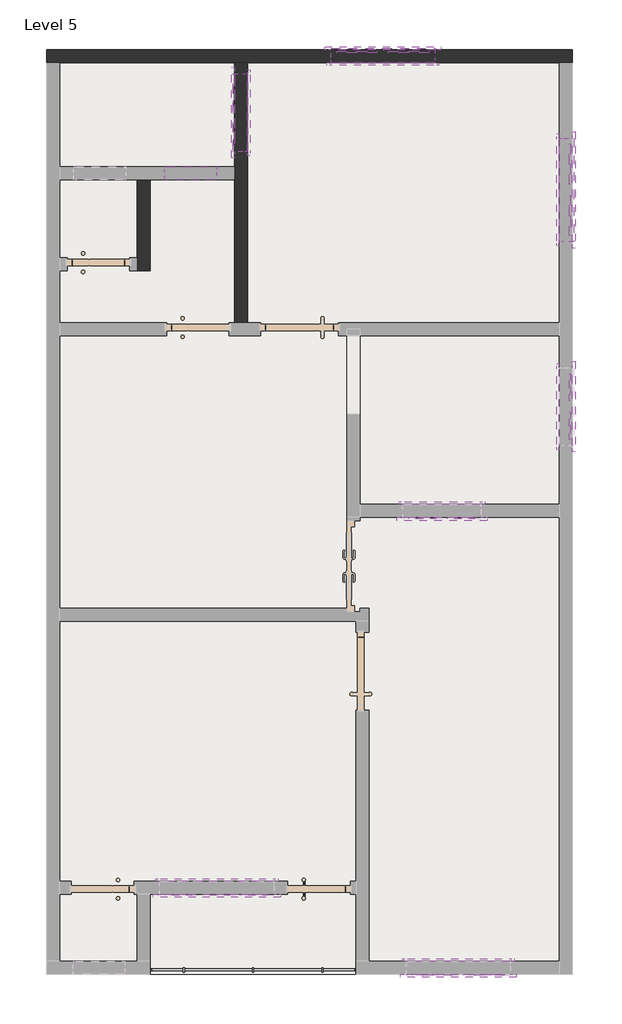
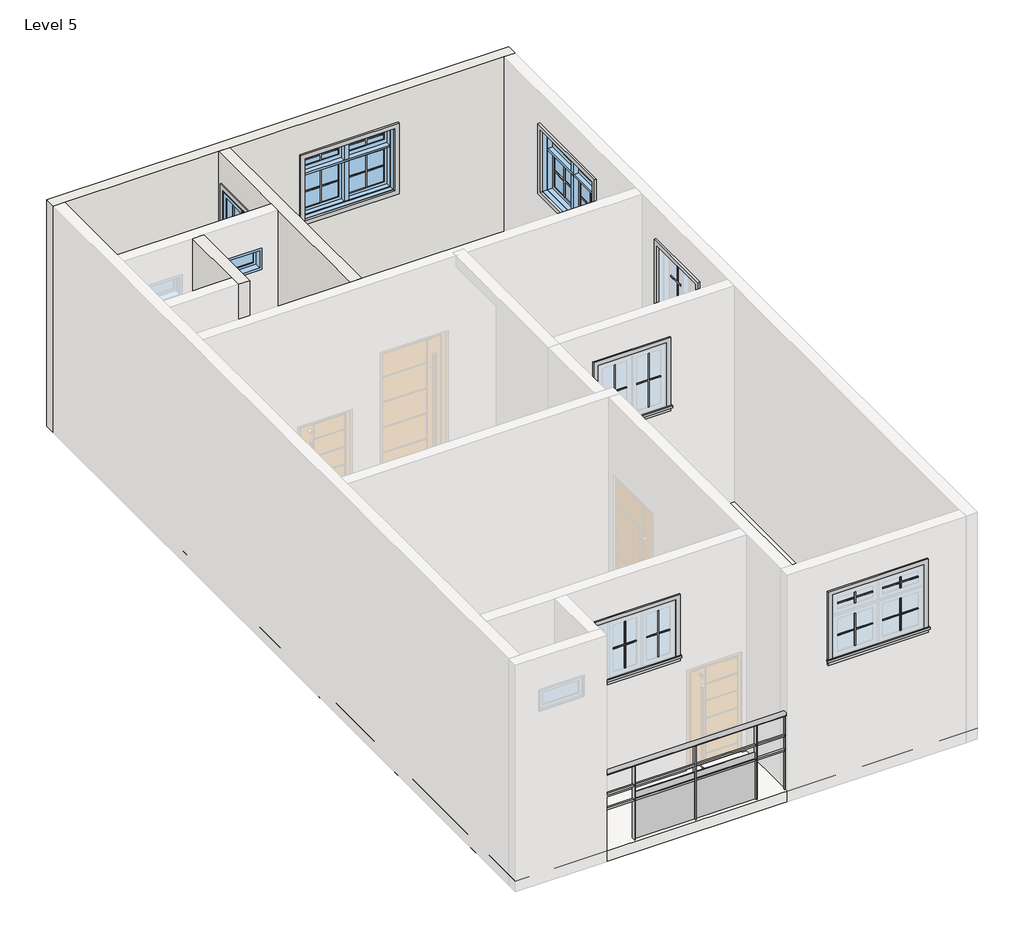
# One storey, part 2 of 2: 35 proxies, 4 windows, 3 walls, 1 railing, 1 slab.
"""IFC4 building model written with IfcOpenShell, lengths in millimetres."""

from ifc_helpers import new_model, si_unit, point, frame, origin, place, context, project, spatial, polyline, ellipse_curve, trimmed, outline, extrude, faceted_brep, transform, mapped, element, save
from ifc_brep_helpers import plane_surface, extruded_surface, advanced_brep
from components import m_muntin_pattern_2x2_m_muntin_pattern_2x2_ec2ff75e, m_muntin_pattern_2x2_m_muntin_pattern_2x2_6a19bea2, m_muntin_pattern_2x2_m_muntin_pattern_2x2_383df7b3, m_muntin_pattern_2x2_m_muntin_pattern_2x2_55460d9e, m_muntin_pattern_2x2_m_muntin_pattern_2x2_a9b7b7a9, m_muntin_pattern_2x2_m_muntin_pattern_2x2_c959817e, m_muntin_pattern_2x2_m_muntin_pattern_2x2_9259c5e2, m_trim_window_exterior_flat_with_sill_b1b88069, m_trim_window_exterior_flat_with_sill_8fa486dc, m_trim_window_exterior_flat_with_sill_2a9c44ae, m_trim_window_interior_flat_picture_frame_7d12f20c, m_trim_window_interior_flat_picture_frame_b6dd03a6, m_trim_window_interior_flat_picture_frame_c139440e, fixed_2_65c13adb, m_window_casement_double_3_e0bd8fa3, m_window_casement_double_awning_double_4_7efa9bbd

model = new_model("IFC4")

# Units and contexts
model_context = context("Model", 3, world=origin())
ifc_project = project(units=[si_unit("LENGTHUNIT", "METRE", prefix="MILLI")], contexts=[model_context])

# Site, building, storey
site = spatial("IfcSite", under=ifc_project)
building = spatial("IfcBuilding", under=site)
storey = spatial("IfcBuildingStorey", under=building, Name="Level 5", Elevation=3810.0)

# Proxies
placement = place(None, origin())
m_muntin_pattern_2x2_m_muntin_pattern_2x2_shape = m_muntin_pattern_2x2_m_muntin_pattern_2x2_ec2ff75e(model_context)
element("IfcBuildingElementProxy", 1, Name="M_Muntin Pattern_2x2 : M_Muntin Pattern_2x2", ObjectType="M_Muntin Pattern_2x2 : M_Muntin Pattern_2x2", at=placement, inside=storey, context=model_context, shape_type="MappedRepresentation", body=[
    mapped(m_muntin_pattern_2x2_m_muntin_pattern_2x2_shape, transform((-20164.8088079, 6316.5492053, 5708.65), x_axis=(1.0, 0.0, 0.0), y_axis=(0.0, 1.0, 0.0), z_axis=(0.0, 0.0, 1.0))),
])
element("IfcBuildingElementProxy", 2, Name="M_Muntin Pattern_2x2 : M_Muntin Pattern_2x2", ObjectType="M_Muntin Pattern_2x2 : M_Muntin Pattern_2x2", at=placement, inside=storey, context=model_context, shape_type="MappedRepresentation", body=[
    mapped(m_muntin_pattern_2x2_m_muntin_pattern_2x2_shape, transform((-17648.6213079, 4984.6367053, 5708.65), x_axis=(0.0, -1.0, 0.0), y_axis=(1.0, 0.0, 0.0), z_axis=(0.0, 0.0, 1.0))),
])
element("IfcBuildingElementProxy", 3, Name="M_Muntin Pattern_2x2 : M_Muntin Pattern_2x2", ObjectType="M_Muntin Pattern_2x2 : M_Muntin Pattern_2x2", at=placement, inside=storey, context=model_context, shape_type="MappedRepresentation", body=[
    mapped(m_muntin_pattern_2x2_m_muntin_pattern_2x2_shape, transform((-18672.7572454, -4510.2007947, 5708.65), x_axis=(-1.0, 0.0, 0.0), y_axis=(0.0, -1.0, 0.0), z_axis=(0.0, 0.0, 1.0))),
])
m_muntin_pattern_2x2_m_muntin_pattern_2x2_2_shape = m_muntin_pattern_2x2_m_muntin_pattern_2x2_6a19bea2(model_context)
element("IfcBuildingElementProxy", 4, Name="M_Muntin Pattern_2x2 : M_Muntin Pattern_2x2", ObjectType="M_Muntin Pattern_2x2 : M_Muntin Pattern_2x2", at=placement, inside=storey, context=model_context, shape_type="MappedRepresentation", body=[
    mapped(m_muntin_pattern_2x2_m_muntin_pattern_2x2_2_shape, transform((-19558.3838079, 6316.5492053, 5708.65), x_axis=(-1.0, 0.0, 0.0), y_axis=(0.0, -1.0, 0.0), z_axis=(0.0, 0.0, 1.0))),
])
element("IfcBuildingElementProxy", 5, Name="M_Muntin Pattern_2x2 : M_Muntin Pattern_2x2", ObjectType="M_Muntin Pattern_2x2 : M_Muntin Pattern_2x2", at=placement, inside=storey, context=model_context, shape_type="MappedRepresentation", body=[
    mapped(m_muntin_pattern_2x2_m_muntin_pattern_2x2_2_shape, transform((-17648.6213079, 4378.2117053, 5708.65), x_axis=(0.0, 1.0, 0.0), y_axis=(-1.0, 0.0, 0.0), z_axis=(0.0, 0.0, 1.0))),
])
element("IfcBuildingElementProxy", 6, Name="M_Muntin Pattern_2x2 : M_Muntin Pattern_2x2", ObjectType="M_Muntin Pattern_2x2 : M_Muntin Pattern_2x2", at=placement, inside=storey, context=model_context, shape_type="MappedRepresentation", body=[
    mapped(m_muntin_pattern_2x2_m_muntin_pattern_2x2_2_shape, transform((-19279.1822454, -4510.2007947, 5708.65), x_axis=(1.0, 0.0, 0.0), y_axis=(0.0, 1.0, 0.0), z_axis=(0.0, 0.0, 1.0))),
])
m_muntin_pattern_2x2_m_muntin_pattern_2x2_3_shape = m_muntin_pattern_2x2_m_muntin_pattern_2x2_383df7b3(model_context)
element("IfcBuildingElementProxy", 7, Name="M_Muntin Pattern_2x2 : M_Muntin Pattern_2x2", ObjectType="M_Muntin Pattern_2x2 : M_Muntin Pattern_2x2", at=placement, inside=storey, context=model_context, shape_type="MappedRepresentation", body=[
    mapped(m_muntin_pattern_2x2_m_muntin_pattern_2x2_3_shape, transform((-19558.3838079, 6316.5492053, 6308.65), x_axis=(-1.0, 0.0, 0.0), y_axis=(0.0, -1.0, 0.0), z_axis=(0.0, 0.0, 1.0))),
])
element("IfcBuildingElementProxy", 8, Name="M_Muntin Pattern_2x2 : M_Muntin Pattern_2x2", ObjectType="M_Muntin Pattern_2x2 : M_Muntin Pattern_2x2", at=placement, inside=storey, context=model_context, shape_type="MappedRepresentation", body=[
    mapped(m_muntin_pattern_2x2_m_muntin_pattern_2x2_3_shape, transform((-20164.8088079, 6316.5492053, 6308.65), x_axis=(-1.0, 0.0, 0.0), y_axis=(0.0, -1.0, 0.0), z_axis=(0.0, 0.0, 1.0))),
])
element("IfcBuildingElementProxy", 9, Name="M_Muntin Pattern_2x2 : M_Muntin Pattern_2x2", ObjectType="M_Muntin Pattern_2x2 : M_Muntin Pattern_2x2", at=placement, inside=storey, context=model_context, shape_type="MappedRepresentation", body=[
    mapped(m_muntin_pattern_2x2_m_muntin_pattern_2x2_3_shape, transform((-17648.6213079, 4378.2117053, 6308.65), x_axis=(0.0, 1.0, 0.0), y_axis=(-1.0, 0.0, 0.0), z_axis=(0.0, 0.0, 1.0))),
])
element("IfcBuildingElementProxy", 10, Name="M_Muntin Pattern_2x2 : M_Muntin Pattern_2x2", ObjectType="M_Muntin Pattern_2x2 : M_Muntin Pattern_2x2", at=placement, inside=storey, context=model_context, shape_type="MappedRepresentation", body=[
    mapped(m_muntin_pattern_2x2_m_muntin_pattern_2x2_3_shape, transform((-17648.6213079, 4984.6367053, 6308.65), x_axis=(0.0, 1.0, 0.0), y_axis=(-1.0, 0.0, 0.0), z_axis=(0.0, 0.0, 1.0))),
])
element("IfcBuildingElementProxy", 11, Name="M_Muntin Pattern_2x2 : M_Muntin Pattern_2x2", ObjectType="M_Muntin Pattern_2x2 : M_Muntin Pattern_2x2", at=placement, inside=storey, context=model_context, shape_type="MappedRepresentation", body=[
    mapped(m_muntin_pattern_2x2_m_muntin_pattern_2x2_3_shape, transform((-19279.1822454, -4510.2007947, 6308.65), x_axis=(1.0, 0.0, 0.0), y_axis=(0.0, 1.0, 0.0), z_axis=(0.0, 0.0, 1.0))),
])
element("IfcBuildingElementProxy", 12, Name="M_Muntin Pattern_2x2 : M_Muntin Pattern_2x2", ObjectType="M_Muntin Pattern_2x2 : M_Muntin Pattern_2x2", at=placement, inside=storey, context=model_context, shape_type="MappedRepresentation", body=[
    mapped(m_muntin_pattern_2x2_m_muntin_pattern_2x2_3_shape, transform((-18672.7572454, -4510.2007947, 6308.65), x_axis=(1.0, 0.0, 0.0), y_axis=(0.0, 1.0, 0.0), z_axis=(0.0, 0.0, 1.0))),
])
m_muntin_pattern_2x2_m_muntin_pattern_2x2_4_shape = m_muntin_pattern_2x2_m_muntin_pattern_2x2_55460d9e(model_context)
element("IfcBuildingElementProxy", 13, Name="M_Muntin Pattern_2x2 : M_Muntin Pattern_2x2", ObjectType="M_Muntin Pattern_2x2 : M_Muntin Pattern_2x2", at=placement, inside=storey, context=model_context, shape_type="MappedRepresentation", body=[
    mapped(m_muntin_pattern_2x2_m_muntin_pattern_2x2_4_shape, transform((-18939.9533391, 849.1992053, 5708.65), x_axis=(-1.0, 0.0, 0.0), y_axis=(0.0, -1.0, 0.0), z_axis=(0.0, 0.0, 1.0))),
])
element("IfcBuildingElementProxy", 14, Name="M_Muntin Pattern_2x2 : M_Muntin Pattern_2x2", ObjectType="M_Muntin Pattern_2x2 : M_Muntin Pattern_2x2", at=placement, inside=storey, context=model_context, shape_type="MappedRepresentation", body=[
    mapped(m_muntin_pattern_2x2_m_muntin_pattern_2x2_4_shape, transform((-17648.6213079, 2366.8492053, 5708.65), x_axis=(0.0, -1.0, 0.0), y_axis=(1.0, 0.0, 0.0), z_axis=(0.0, 0.0, 1.0))),
])
element("IfcBuildingElementProxy", 15, Name="M_Muntin Pattern_2x2 : M_Muntin Pattern_2x2", ObjectType="M_Muntin Pattern_2x2 : M_Muntin Pattern_2x2", at=placement, inside=storey, context=model_context, shape_type="MappedRepresentation", body=[
    mapped(m_muntin_pattern_2x2_m_muntin_pattern_2x2_4_shape, transform((-21591.9713079, 5362.4617053, 5708.65), x_axis=(0.0, 1.0, 0.0), y_axis=(-1.0, 0.0, 0.0), z_axis=(0.0, 0.0, 1.0))),
])
m_muntin_pattern_2x2_m_muntin_pattern_2x2_5_shape = m_muntin_pattern_2x2_m_muntin_pattern_2x2_a9b7b7a9(model_context)
element("IfcBuildingElementProxy", 16, Name="M_Muntin Pattern_2x2 : M_Muntin Pattern_2x2", ObjectType="M_Muntin Pattern_2x2 : M_Muntin Pattern_2x2", at=placement, inside=storey, context=model_context, shape_type="MappedRepresentation", body=[
    mapped(m_muntin_pattern_2x2_m_muntin_pattern_2x2_5_shape, transform((-19393.9783391, 849.1992053, 5708.65), x_axis=(1.0, 0.0, 0.0), y_axis=(0.0, 1.0, 0.0), z_axis=(0.0, 0.0, 1.0))),
])
element("IfcBuildingElementProxy", 17, Name="M_Muntin Pattern_2x2 : M_Muntin Pattern_2x2", ObjectType="M_Muntin Pattern_2x2 : M_Muntin Pattern_2x2", at=placement, inside=storey, context=model_context, shape_type="MappedRepresentation", body=[
    mapped(m_muntin_pattern_2x2_m_muntin_pattern_2x2_5_shape, transform((-17648.6213079, 1912.8242053, 5708.65), x_axis=(0.0, 1.0, 0.0), y_axis=(-1.0, 0.0, 0.0), z_axis=(0.0, 0.0, 1.0))),
])
element("IfcBuildingElementProxy", 18, Name="M_Muntin Pattern_2x2 : M_Muntin Pattern_2x2", ObjectType="M_Muntin Pattern_2x2 : M_Muntin Pattern_2x2", at=placement, inside=storey, context=model_context, shape_type="MappedRepresentation", body=[
    mapped(m_muntin_pattern_2x2_m_muntin_pattern_2x2_5_shape, transform((-21591.9713079, 5816.4867053, 5708.65), x_axis=(0.0, -1.0, 0.0), y_axis=(1.0, 0.0, 0.0), z_axis=(0.0, 0.0, 1.0))),
])
m_muntin_pattern_2x2_m_muntin_pattern_2x2_6_shape = m_muntin_pattern_2x2_m_muntin_pattern_2x2_c959817e(model_context)
element("IfcBuildingElementProxy", 19, Name="M_Muntin Pattern_2x2 : M_Muntin Pattern_2x2", ObjectType="M_Muntin Pattern_2x2 : M_Muntin Pattern_2x2", at=placement, inside=storey, context=model_context, shape_type="MappedRepresentation", body=[
    mapped(m_muntin_pattern_2x2_m_muntin_pattern_2x2_6_shape, transform((-21364.4296412, -3570.4007947, 5708.65), x_axis=(-1.0, 0.0, 0.0), y_axis=(0.0, -1.0, 0.0), z_axis=(0.0, 0.0, 1.0))),
])
m_muntin_pattern_2x2_m_muntin_pattern_2x2_7_shape = m_muntin_pattern_2x2_m_muntin_pattern_2x2_9259c5e2(model_context)
element("IfcBuildingElementProxy", 20, Name="M_Muntin Pattern_2x2 : M_Muntin Pattern_2x2", ObjectType="M_Muntin Pattern_2x2 : M_Muntin Pattern_2x2", at=placement, inside=storey, context=model_context, shape_type="MappedRepresentation", body=[
    mapped(m_muntin_pattern_2x2_m_muntin_pattern_2x2_7_shape, transform((-22257.6629746, -3570.4007947, 5708.65), x_axis=(1.0, 0.0, 0.0), y_axis=(0.0, 1.0, 0.0), z_axis=(0.0, 0.0, 1.0))),
])
element("IfcBuildingElementProxy", 21, Name="M_Muntin Pattern_2x2 : M_Muntin Pattern_2x2", ObjectType="M_Muntin Pattern_2x2 : M_Muntin Pattern_2x2", at=placement, inside=storey, context=model_context, shape_type="MappedRepresentation", body=[
    mapped(m_muntin_pattern_2x2_m_muntin_pattern_2x2_7_shape, transform((-21811.0463079, -3570.4007947, 5708.65), x_axis=(1.0, 0.0, 0.0), y_axis=(0.0, 1.0, 0.0), z_axis=(0.0, 0.0, 1.0))),
])
m_trim_window_exterior_flat_with_sill_shape = m_trim_window_exterior_flat_with_sill_b1b88069(model_context)
element("IfcBuildingElementProxy", 22, Name="M_Trim-Window-Exterior-Flat : with Sill", ObjectType="M_Trim-Window-Exterior-Flat : with Sill", at=placement, inside=storey, context=model_context, shape_type="MappedRepresentation", body=[
    mapped(m_trim_window_exterior_flat_with_sill_shape, transform((-19861.5963079, 6326.0742053, 6538.8), x_axis=(-1.0, 0.0, 0.0), y_axis=(0.0, 0.0, 1.0), z_axis=(0.0, 1.0, 0.0))),
])
element("IfcBuildingElementProxy", 23, Name="M_Trim-Window-Exterior-Flat : with Sill", ObjectType="M_Trim-Window-Exterior-Flat : with Sill", at=placement, inside=storey, context=model_context, shape_type="MappedRepresentation", body=[
    mapped(m_trim_window_exterior_flat_with_sill_shape, transform((-17639.0963079, 4681.4242053, 6538.8), x_axis=(0.0, 1.0, 0.0), y_axis=(0.0, 0.0, 1.0), z_axis=(1.0, 0.0, 0.0))),
])
element("IfcBuildingElementProxy", 24, Name="M_Trim-Window-Exterior-Flat : with Sill", ObjectType="M_Trim-Window-Exterior-Flat : with Sill", at=placement, inside=storey, context=model_context, shape_type="MappedRepresentation", body=[
    mapped(m_trim_window_exterior_flat_with_sill_shape, transform((-18975.9697454, -4519.7257947, 6538.8), x_axis=(1.0, 0.0, 0.0), y_axis=(0.0, 0.0, 1.0), z_axis=(0.0, -1.0, 0.0))),
])
m_trim_window_exterior_flat_with_sill_2_shape = m_trim_window_exterior_flat_with_sill_8fa486dc(model_context)
element("IfcBuildingElementProxy", 25, Name="M_Trim-Window-Exterior-Flat : with Sill", ObjectType="M_Trim-Window-Exterior-Flat : with Sill", at=placement, inside=storey, context=model_context, shape_type="MappedRepresentation", body=[
    mapped(m_trim_window_exterior_flat_with_sill_2_shape, transform((-19166.9658391, 839.6742053, 6538.8), x_axis=(1.0, 0.0, 0.0), y_axis=(0.0, 0.0, 1.0), z_axis=(0.0, -1.0, 0.0))),
])
element("IfcBuildingElementProxy", 26, Name="M_Trim-Window-Exterior-Flat : with Sill", ObjectType="M_Trim-Window-Exterior-Flat : with Sill", at=placement, inside=storey, context=model_context, shape_type="MappedRepresentation", body=[
    mapped(m_trim_window_exterior_flat_with_sill_2_shape, transform((-17639.0963079, 2139.8367053, 6538.8), x_axis=(0.0, 1.0, 0.0), y_axis=(0.0, 0.0, 1.0), z_axis=(1.0, 0.0, 0.0))),
])
element("IfcBuildingElementProxy", 27, Name="M_Trim-Window-Exterior-Flat : with Sill", ObjectType="M_Trim-Window-Exterior-Flat : with Sill", at=placement, inside=storey, context=model_context, shape_type="MappedRepresentation", body=[
    mapped(m_trim_window_exterior_flat_with_sill_2_shape, transform((-21601.4963079, 5589.4742053, 6538.8), x_axis=(0.0, -1.0, 0.0), y_axis=(0.0, 0.0, 1.0), z_axis=(-1.0, 0.0, 0.0))),
])
m_trim_window_exterior_flat_with_sill_3_shape = m_trim_window_exterior_flat_with_sill_2a9c44ae(model_context)
element("IfcBuildingElementProxy", 28, Name="M_Trim-Window-Exterior-Flat : with Sill", ObjectType="M_Trim-Window-Exterior-Flat : with Sill", at=placement, inside=storey, context=model_context, shape_type="MappedRepresentation", body=[
    mapped(m_trim_window_exterior_flat_with_sill_3_shape, transform((-21811.0463079, -3579.9257947, 6438.8), x_axis=(1.0, 0.0, 0.0), y_axis=(0.0, 0.0, 1.0), z_axis=(0.0, -1.0, 0.0))),
])
m_trim_window_interior_flat_picture_frame_shape = m_trim_window_interior_flat_picture_frame_7d12f20c(model_context)
element("IfcBuildingElementProxy", 29, Name="M_Trim-Window-Interior-Flat : Picture Frame", ObjectType="M_Trim-Window-Interior-Flat : Picture Frame", at=placement, inside=storey, context=model_context, shape_type="MappedRepresentation", body=[
    mapped(m_trim_window_interior_flat_picture_frame_shape, transform((-19861.5963079, 6173.6742053, 6538.8), x_axis=(1.0, 0.0, 0.0), y_axis=(0.0, 0.0, 1.0), z_axis=(0.0, -1.0, 0.0))),
])
element("IfcBuildingElementProxy", 30, Name="M_Trim-Window-Interior-Flat : Picture Frame", ObjectType="M_Trim-Window-Interior-Flat : Picture Frame", at=placement, inside=storey, context=model_context, shape_type="MappedRepresentation", body=[
    mapped(m_trim_window_interior_flat_picture_frame_shape, transform((-17791.4963079, 4681.4242053, 6538.8), x_axis=(0.0, -1.0, 0.0), y_axis=(0.0, 0.0, 1.0), z_axis=(-1.0, 0.0, 0.0))),
])
element("IfcBuildingElementProxy", 31, Name="M_Trim-Window-Interior-Flat : Picture Frame", ObjectType="M_Trim-Window-Interior-Flat : Picture Frame", at=placement, inside=storey, context=model_context, shape_type="MappedRepresentation", body=[
    mapped(m_trim_window_interior_flat_picture_frame_shape, transform((-18975.9697454, -4367.3257947, 6538.8), x_axis=(-1.0, 0.0, 0.0), y_axis=(0.0, 0.0, 1.0), z_axis=(0.0, 1.0, 0.0))),
])
m_trim_window_interior_flat_picture_frame_2_shape = m_trim_window_interior_flat_picture_frame_b6dd03a6(model_context)
element("IfcBuildingElementProxy", 32, Name="M_Trim-Window-Interior-Flat : Picture Frame", ObjectType="M_Trim-Window-Interior-Flat : Picture Frame", at=placement, inside=storey, context=model_context, shape_type="MappedRepresentation", body=[
    mapped(m_trim_window_interior_flat_picture_frame_2_shape, transform((-19166.9658391, 992.0742053, 6538.8), x_axis=(-1.0, 0.0, 0.0), y_axis=(0.0, 0.0, 1.0), z_axis=(0.0, 1.0, 0.0))),
])
element("IfcBuildingElementProxy", 33, Name="M_Trim-Window-Interior-Flat : Picture Frame", ObjectType="M_Trim-Window-Interior-Flat : Picture Frame", at=placement, inside=storey, context=model_context, shape_type="MappedRepresentation", body=[
    mapped(m_trim_window_interior_flat_picture_frame_2_shape, transform((-17791.4963079, 2139.8367053, 6538.8), x_axis=(0.0, -1.0, 0.0), y_axis=(0.0, 0.0, 1.0), z_axis=(-1.0, 0.0, 0.0))),
])
element("IfcBuildingElementProxy", 34, Name="M_Trim-Window-Interior-Flat : Picture Frame", ObjectType="M_Trim-Window-Interior-Flat : Picture Frame", at=placement, inside=storey, context=model_context, shape_type="MappedRepresentation", body=[
    mapped(m_trim_window_interior_flat_picture_frame_2_shape, transform((-21449.0963079, 5589.4742053, 6538.8), x_axis=(0.0, 1.0, 0.0), y_axis=(0.0, 0.0, 1.0), z_axis=(1.0, 0.0, 0.0))),
])
m_trim_window_interior_flat_picture_frame_3_shape = m_trim_window_interior_flat_picture_frame_c139440e(model_context)
element("IfcBuildingElementProxy", 35, Name="M_Trim-Window-Interior-Flat : Picture Frame", ObjectType="M_Trim-Window-Interior-Flat : Picture Frame", at=placement, inside=storey, context=model_context, shape_type="MappedRepresentation", body=[
    mapped(m_trim_window_interior_flat_picture_frame_3_shape, transform((-21811.0463079, -3427.5257947, 6438.8), x_axis=(-1.0, 0.0, 0.0), y_axis=(0.0, 0.0, 1.0), z_axis=(0.0, 1.0, 0.0))),
])

# Railing
element("IfcRailing", 36, ObjectType="Glass Panel - Bottom Fill", at=placement, inside=storey, context=model_context, shape_type="SolidModel", body=[
    advanced_brep(
    [(-22592.0963079, -4430.8257947, 5029.2), (-22592.0963079, -4507.0257947, 5029.2), (-20179.0963079, -4430.8257947, 5029.2), (-20179.0963079, -4507.0257947, 5029.2)],
    [
        (0, 1, ellipse_curve(frame((-22592.0963079, -4468.9257947, 5029.2), z_axis=(-1.0, 0.0, 0.0), x_axis=(0.0, -1.0, 0.0)), 38.1, 28.575)),
        (1, 0, ellipse_curve(frame((-22592.0963079, -4468.9257947, 5029.2), z_axis=(-1.0, 0.0, 0.0), x_axis=(0.0, -1.0, 0.0)), 38.1, 28.575)),
        (2, 3, ellipse_curve(frame((-20179.0963079, -4468.9257947, 5029.2), z_axis=(1.0, 0.0, 0.0), x_axis=(0.0, -1.0, 0.0)), 38.1, 28.575)),
        (3, 2, ellipse_curve(frame((-20179.0963079, -4468.9257947, 5029.2), z_axis=(1.0, 0.0, 0.0), x_axis=(0.0, -1.0, 0.0)), 38.1, 28.575)),
        (0, 2),
        (3, 1),
    ],
    [
        plane_surface(frame((-22592.0963079, -4468.9257947, 5029.2), z_axis=(-1.0, 0.0, 0.0), x_axis=(0.0, 1.0, 0.0))),
        plane_surface(frame((-20179.0963079, -4468.9257947, 5029.2), z_axis=(1.0, 0.0, 0.0), x_axis=(0.0, 1.0, 0.0))),
        extruded_surface(trimmed(ellipse_curve(frame((-20179.0963079, -4468.9257947, 5029.2), z_axis=(-1.0, 0.0, 0.0), x_axis=(0.0, -1.0, 0.0)), 38.1, 28.575), [point((-20179.0963079, -4430.8257947, 5029.2))], [point((-20179.0963079, -4507.0257947, 5029.2))], True, "CARTESIAN"), (-2413.0, 0.0, 0.0), 2413.0),
        extruded_surface(trimmed(ellipse_curve(frame((-20179.0963079, -4468.9257947, 5029.2), z_axis=(-1.0, 0.0, 0.0), x_axis=(0.0, -1.0, 0.0)), 38.1, 28.575), [point((-20179.0963079, -4507.0257947, 5029.2))], [point((-20179.0963079, -4430.8257947, 5029.2))], True, "CARTESIAN"), (-2413.0, 0.0, 0.0), 2413.0),
    ],
    [
        (0, [[1, 2]]),
        (1, [[3, 4]]),
        (2, [[-1, 5, -4, 6]]),
        (3, [[-2, -6, -3, -5]]),
    ],
),
    extrude(outline(polyline([(-22592.0963079, -4481.6257947), (-22592.0963079, -4456.2257947), (-20179.0963079, -4456.2257947), (-20179.0963079, -4481.6257947), (-22592.0963079, -4481.6257947)])), frame((0.0, 0.0, 4711.7), z_axis=(0.0, 0.0, 1.0), x_axis=(1.0, 0.0, 0.0)), (0.0, 0.0, 1.0), 25.4),
    extrude(outline(polyline([(-22592.0963079, -4481.6257947), (-22592.0963079, -4456.2257947), (-20179.0963079, -4456.2257947), (-20179.0963079, -4481.6257947), (-22592.0963079, -4481.6257947)])), frame((0.0, 0.0, 4508.5), z_axis=(0.0, 0.0, 1.0), x_axis=(1.0, 0.0, 0.0)), (0.0, 0.0, 1.0), 25.4),
    extrude(outline(polyline([(-20579.1463079, -4494.3257947), (-20579.1463079, -4443.5257947), (-20566.4463079, -4443.5257947), (-20566.4463079, -4494.3257947), (-20579.1463079, -4494.3257947)])), frame((0.0, 0.0, 3810.0), z_axis=(0.0, 0.0, 1.0), x_axis=(1.0, 0.0, 0.0)), (0.0, 0.0, 1.0), 1190.625),
    extrude(outline(polyline([(-21385.5963079, -4462.3906377), (-20572.7963079, -4462.3906377), (-20572.7963079, -4468.7406377), (-21385.5963079, -4468.7406377), (-21385.5963079, -4462.3906377)])), frame((0.0, 0.0, 3911.6), z_axis=(0.0, 0.0, 1.0), x_axis=(1.0, 0.0, 0.0)), (0.0, 0.0, 1.0), 711.2),
    extrude(outline(polyline([(-21391.9463079, -4494.3257947), (-21391.9463079, -4443.5257947), (-21379.2463079, -4443.5257947), (-21379.2463079, -4494.3257947), (-21391.9463079, -4494.3257947)])), frame((0.0, 0.0, 3810.0), z_axis=(0.0, 0.0, 1.0), x_axis=(1.0, 0.0, 0.0)), (0.0, 0.0, 1.0), 1190.625),
    extrude(outline(polyline([(-22198.3963079, -4462.3906377), (-21385.5963079, -4462.3906377), (-21385.5963079, -4468.7406377), (-22198.3963079, -4468.7406377), (-22198.3963079, -4462.3906377)])), frame((0.0, 0.0, 3911.6), z_axis=(0.0, 0.0, 1.0), x_axis=(1.0, 0.0, 0.0)), (0.0, 0.0, 1.0), 711.2),
    extrude(outline(polyline([(-22204.7463079, -4494.3257947), (-22204.7463079, -4443.5257947), (-22192.0463079, -4443.5257947), (-22192.0463079, -4494.3257947), (-22204.7463079, -4494.3257947)])), frame((0.0, 0.0, 3810.0), z_axis=(0.0, 0.0, 1.0), x_axis=(1.0, 0.0, 0.0)), (0.0, 0.0, 1.0), 1190.625),
    extrude(outline(polyline([(-20191.7963079, -4478.4507947), (-20191.7963079, -4459.4007947), (-20172.7463079, -4459.4007947), (-20172.7463079, -4478.4507947), (-20191.7963079, -4478.4507947)])), frame((0.0, 0.0, 3810.0), z_axis=(0.0, 0.0, 1.0), x_axis=(1.0, 0.0, 0.0)), (0.0, 0.0, 1.0), 1190.625),
    extrude(outline(polyline([(-22598.4463079, -4478.4507947), (-22598.4463079, -4459.4007947), (-22579.3963079, -4459.4007947), (-22579.3963079, -4478.4507947), (-22598.4463079, -4478.4507947)])), frame((0.0, 0.0, 3810.0), z_axis=(0.0, 0.0, 1.0), x_axis=(1.0, 0.0, 0.0)), (0.0, 0.0, 1.0), 1190.625),
])

# Slab
element("IfcSlab", 37, ObjectType="Generic - 6\"", at=placement, inside=storey, context=model_context, shape_type="SweptSolid", body=[
    extrude(outline(polyline([(-23811.2963079, -4519.7257947), (-23811.2963079, 6326.0742053), (-17639.0963079, 6326.0742053), (-17639.0963079, -4519.7257947), (-23811.2963079, -4519.7257947)])), frame((0.0, 0.0, 3810.0), z_axis=(0.0, 0.0, 1.0), x_axis=(1.0, 0.0, 0.0)), (0.0, 0.0, 1.0), 152.4),
])

# Walls
element("IfcWall", 38, ObjectType="Generic - 6\"", at=placement, inside=storey, context=model_context, shape_type="Brep", body=[
    faceted_brep([(-23811.2963079, 6173.6742053, 3810.0), (-23658.8963079, 6173.6742053, 3810.0), (-21601.4963079, 6173.6742053, 3810.0), (-21449.0963079, 6173.6742053, 3810.0), (-17791.4963079, 6173.6742053, 3810.0), (-17639.0963079, 6173.6742053, 3810.0), (-17639.0963079, 6173.6742053, 7010.4), (-17791.4963079, 6173.6742053, 7010.4), (-21449.0963079, 6173.6742053, 7010.4), (-21601.4963079, 6173.6742053, 7010.4), (-23658.8963079, 6173.6742053, 7010.4), (-23811.2963079, 6173.6742053, 7010.4), (-19251.9963079, 6173.6742053, 6538.8), (-19251.9963079, 6173.6742053, 5638.8), (-20471.1963079, 6173.6742053, 5638.8), (-20471.1963079, 6173.6742053, 6538.8), (-23811.2963079, 6326.0742053, 3810.0), (-23811.2963079, 6326.0742053, 7010.4), (-17639.0963079, 6326.0742053, 7010.4), (-17639.0963079, 6326.0742053, 3810.0), (-19251.9963079, 6326.0742053, 6538.8), (-20471.1963079, 6326.0742053, 6538.8), (-20471.1963079, 6326.0742053, 5638.8), (-19251.9963079, 6326.0742053, 5638.8)], [[[0, 1, 2, 3, 4, 5, 6, 7, 8, 9, 10, 11], [12, 13, 14, 15]], [[16, 17, 18, 19], [20, 21, 22, 23]], [[5, 4, 3, 2, 1, 0, 16, 19]], [[11, 10, 9, 8, 7, 6, 18, 17]], [[6, 5, 19, 18]], [[0, 11, 17, 16]], [[13, 12, 20, 23]], [[14, 13, 23, 22]], [[15, 14, 22, 21]], [[12, 15, 21, 20]]]),
])
element("IfcWall", 39, ObjectType="Generic - 6\"", at=placement, inside=storey, context=model_context, shape_type="Brep", body=[
    faceted_brep([(-21601.4963079, 6173.6742053, 3810.0), (-21601.4963079, 4954.4742053, 3810.0), (-21601.4963079, 4802.0742053, 3810.0), (-21601.4963079, 3125.6742053, 3810.0), (-21601.4963079, 3125.6742053, 7010.4), (-21601.4963079, 4802.0742053, 7010.4), (-21601.4963079, 4954.4742053, 7010.4), (-21601.4963079, 6173.6742053, 7010.4), (-21601.4963079, 6046.6742053, 6538.8), (-21601.4963079, 5132.2742053, 6538.8), (-21601.4963079, 5132.2742053, 5638.8), (-21601.4963079, 6046.6742053, 5638.8), (-21449.0963079, 6173.6742053, 3810.0), (-21449.0963079, 6173.6742053, 7010.4), (-21449.0963079, 3125.6742053, 7010.4), (-21449.0963079, 3125.6742053, 3810.0), (-21449.0963079, 6046.6742053, 6538.8), (-21449.0963079, 6046.6742053, 5638.8), (-21449.0963079, 5132.2742053, 5638.8), (-21449.0963079, 5132.2742053, 6538.8)], [[[0, 1, 2, 3, 4, 5, 6, 7], [8, 9, 10, 11]], [[12, 13, 14, 15], [16, 17, 18, 19]], [[3, 2, 1, 0, 12, 15]], [[7, 6, 5, 4, 14, 13]], [[0, 7, 13, 12]], [[4, 3, 15, 14]], [[17, 16, 8, 11]], [[18, 17, 11, 10]], [[19, 18, 10, 9]], [[16, 19, 9, 8]]]),
])
element("IfcWall", 40, ObjectType="Generic - 6\"", at=placement, inside=storey, context=model_context, shape_type="Brep", body=[
    faceted_brep([(-22744.4963079, 4802.0742053, 3810.0), (-22744.4963079, 3887.6742053, 3810.0), (-22744.4963079, 3735.2742053, 3810.0), (-22744.4963079, 3735.2742053, 7010.4), (-22744.4963079, 3887.6742053, 7010.4), (-22744.4963079, 4802.0742053, 7010.4), (-22592.0963079, 4802.0742053, 3810.0), (-22592.0963079, 4802.0742053, 7010.4), (-22592.0963079, 3735.2742053, 7010.4), (-22592.0963079, 3735.2742053, 3810.0)], [[[0, 1, 2, 3, 4, 5]], [[6, 7, 8, 9]], [[2, 1, 0, 6, 9]], [[5, 4, 3, 8, 7]], [[0, 5, 7, 6]], [[3, 2, 9, 8]]]),
])

# Windows
fixed_2_shape = fixed_2_65c13adb(model_context)
element("IfcWindow", 41, ObjectType="Fixed : 2'", at=placement, inside=storey, context=model_context, shape_type="MappedRepresentation", body=[
    mapped(fixed_2_shape, transform((-22079.3338079, 4878.2742053, 5334.0), x_axis=(1.0, 0.0, 0.0), y_axis=(0.0, 1.0, 0.0), z_axis=(0.0, 0.0, 1.0))),
])
m_window_casement_double_3_shape = m_window_casement_double_3_e0bd8fa3(model_context)
element("IfcWindow", 42, ObjectType="M_Window-Casement-Double : 3'", at=placement, inside=storey, context=model_context, shape_type="MappedRepresentation", body=[
    mapped(m_window_casement_double_3_shape, transform((-21525.2963079, 5589.4742053, 4738.8), x_axis=(0.0, 1.0, 0.0), y_axis=(-1.0, 0.0, 0.0), z_axis=(0.0, 0.0, 1.0))),
])
m_window_casement_double_awning_double_4_shape = m_window_casement_double_awning_double_4_7efa9bbd(model_context)
element("IfcWindow", 43, ObjectType="M_Window-Casement-Double-Awning-Double : 4'", at=placement, inside=storey, context=model_context, shape_type="MappedRepresentation", body=[
    mapped(m_window_casement_double_awning_double_4_shape, transform((-19861.5963079, 6249.8742053, 4738.8), x_axis=(1.0, 0.0, 0.0), y_axis=(0.0, 1.0, 0.0), z_axis=(0.0, 0.0, 1.0))),
])
element("IfcWindow", 44, ObjectType="M_Window-Casement-Double-Awning-Double : 4'", at=placement, inside=storey, context=model_context, shape_type="MappedRepresentation", body=[
    mapped(m_window_casement_double_awning_double_4_shape, transform((-17715.2963079, 4681.4242053, 4738.8), x_axis=(0.0, -1.0, 0.0), y_axis=(1.0, 0.0, 0.0), z_axis=(0.0, 0.0, 1.0))),
])

save(model, "model.ifc")

# Revit data of these elements
# Type "M_Muntin Pattern_2x2 : M_Muntin Pattern_2x2"
#   Width [instance default] = 3' - 11.24409"
#   Thickness = 0' - 0 1/2"
#   Height [instance default] = 3' - 11.24409"
#   Distance = 0' - 0 3/4"
#   Interior Material [instance default] = none
#   Exterior Material [instance default] = none
#   Default Elevation = 0
# Type "M_Trim-Window-Exterior-Flat : with Sill"
#   Trim Width = 0' - 2.3622"
#   Trim Thickness_Picture Frame = 0' - 1.1811"
#   Trim Thickness_with Sill = 0' - 0 3/4"
#   Sill Thickness = 0' - 1.1811"
#   Opening Width [instance default] = 1' - 11.62205"
#   Opening Height [instance default] = 2' - 11.43307"
#   Default Elevation = 3' - 11.24409"
#   Sill = yes
#   Picture Frame = no
#   Trim Material [instance default] = none
# Type "M_Trim-Window-Interior-Flat : Picture Frame"
#   Trim Thickness_Picture Frame = 0' - 1.1811"
#   Trim Width = 0' - 2.3622"
#   Trim Thickness_with Sill = 0' - 0.7874"
#   Sill Thickness = 0' - 1.1811"
#   Opening Width [instance default] = 1' - 11.62205"
#   Opening Height [instance default] = 2' - 11.43307"
#   Default Elevation = 3' - 11.24409"
#   Sill = no
#   Picture Frame = yes
#   Trim Material [instance default] = none
# Type "Glass Panel - Bottom Fill"
#   Assembly Code = "C2010400"
#   built-in parameter 1008612 = 0.0416667 (stored number, unit not read)
#   built-in parameter 1008611 = 0.0416667 (stored number, unit not read)
#   built-in parameter 1008609 = 0.333333 (stored number, unit not read)
#   built-in parameter 1008604 = 0.166667 (stored number, unit not read)
#   built-in parameter 1008603 = 0.166667 (stored number, unit not read)
#   Railing Height = 4' - 0"
#   built-in parameter 1008630 = 2
#   built-in parameter 1008610 = 2
#   built-in parameter 1008618 = Baluster - Square : 3/4"
# Type "Generic - 6\""
#   Assembly Code = "B1010"
#   Function = 0
#   Layers, outside or top first: 0' - 6" no material (function 1)
# Type "Generic - 6\""
#   Assembly Code = "B2010"
#   Layers, outside or top first: 0' - 6" no material (function 1)
# Type "Fixed : 2'"
#   Type Mark = "16"
#   Assembly Code = "B2020100"
#   Height = 1' - 0"
#   Default Sill Height = 3' - 0"
#   Width = 2' - 0"
#   Window Inset = 0' - 0 3/4"
#   Glass Pane Material = Glass
#   Sash Material = Sash
#   Wall Closure = (empty or 0)
# Type "M_Window-Casement-Double : 3'"
#   Type Mark = "13"
#   Fire Rating = "0.5h"
#   Assembly Code = "B2020100"
#   Analytic Construction = "Double glazing - domestic"
#   Frame Extension [instance default] = 0' - 0 1/4"
#   Window Inset [instance default] = 0' - 0"
#   Wall Thickness [instance default] = 0' - 5.90551"
#   Interior Wall Closure [instance default] = 0' - 2.15551"
#   Half Width = 1' - 6"
#   Visual Light Transmittance = 0.81
#   Thermal Resistance (R) = 1.8146 (h·ft²·°F)/BTU
#   Solar Heat Gain Coefficient = 0.76
#   Rough Width = 3' - 0.59055"
#   Rough Height = 3' - 0.02362"
#   Height = 2' - 11.43307"
#   Heat Transfer Coefficient (U) = 0.5511 BTU/(h·ft²·°F)
#   Exterior Wall Closure [instance default] = 0' - 1.25197"
#   Extension Jamb [instance default] = 0' - 2.15551"
#   Default Sill Height = 2' - 11.43307"
#   Width = 3' - 0"
#   Muntin Visibility = yes
#   Interior Trim Visibility [instance default] = yes
#   Exterior Trim Visibility [instance default] = yes
#   Extension Jamb Visibility [instance default] = yes
#   Interior Trim Material = Wood - Stained
#   Muntin Pattern = M_Muntin Pattern_2x2 : M_Muntin Pattern_2x2
#   Interior Trim = M_Trim-Window-Interior-Flat : Picture Frame
#   Interior Frame Material = Wood - Stained
#   Glass Panel Material = Glass
#   Exterior Trim Material = Clad - White
#   Exterior Trim = M_Trim-Window-Exterior-Flat : with Sill
#   Exterior Frame Material = Clad - White
#   Wall Closure = (empty or 0)
# Type "M_Window-Casement-Double-Awning-Double : 4'"
#   Type Mark = "11"
#   Fire Rating = "0.5h"
#   Assembly Code = "B2020100"
#   Analytic Construction = "Double glazing - domestic"
#   Window Inset [instance default] = 0' - 0"
#   Wall Thickness [instance default] = 0' - 5.90551"
#   Interior Wall Closure [instance default] = 0' - 2.15551"
#   Half Width = 2' - 0"
#   Visual Light Transmittance = 0.81
#   Transom Height = 0' - 11.81102"
#   Thermal Resistance (R) = 1.8146 (h·ft²·°F)/BTU
#   Solar Heat Gain Coefficient = 0.76
#   Rough Width = 4' - 0.59055"
#   Rough Height = 3' - 0.02362"
#   Open Window Height = 1' - 11.62205"
#   Frame Extension [instance default] = 0' - 0 1/4"
#   Height = 2' - 11.43307"
#   Heat Transfer Coefficient (U) = 0.5511 BTU/(h·ft²·°F)
#   Exterior Wall Closure [instance default] = 0' - 1.25197"
#   Extension Jamb [instance default] = 0' - 2.15551"
#   Default Sill Height = 2' - 11.43307"
#   Width = 4' - 0"
#   Top Muntin Visibility = yes
#   Bottom Muntin Visibility = yes
#   Interior Trim Visibility [instance default] = yes
#   Exterior Trim Visibility [instance default] = yes
#   Extension Jamb Visibility [instance default] = yes
#   Interior Trim Material = Wood - Stained
#   Muntin Pattern = M_Muntin Pattern_2x2 : M_Muntin Pattern_2x2
#   Interior Trim = M_Trim-Window-Interior-Flat : Picture Frame
#   Interior Frame Material = Wood - Stained
#   Glass Panel Material = Glass
#   Exterior Trim Material = Clad - White
#   Exterior Trim = M_Trim-Window-Exterior-Flat : with Sill
#   Exterior Frame Material = Clad - White
#   Wall Closure = (empty or 0)
# Elements 1, 2, 3, 4, 5, 6 (IfcBuildingElementProxy, "M_Muntin Pattern_2x2 : M_Muntin Pattern_2x2")
#   Width = 1' - 6 5/8"
#   Height = 1' - 6.12205"
#   Interior Material = Wood - Stained
#   Exterior Material = Clad - White
#   Phase Created = New Construction
#   Materials on its faces: "Clad - White", "Wood - Stained"
# Elements 7, 8, 9, 10, 11, 12 (IfcBuildingElementProxy, "M_Muntin Pattern_2x2 : M_Muntin Pattern_2x2")
#   Width = 1' - 6 5/8"
#   Height = 0' - 6.31102"
#   Interior Material = Wood - Stained
#   Exterior Material = Clad - White
#   Phase Created = New Construction
#   Materials on its faces: "Clad - White", "Wood - Stained"
# Elements 13, 14, 15, 16, 17, 18 (IfcBuildingElementProxy, "M_Muntin Pattern_2x2 : M_Muntin Pattern_2x2")
#   Width = 1' - 0 5/8"
#   Height = 2' - 5.93307"
#   Interior Material = Wood - Stained
#   Exterior Material = Clad - White
#   Phase Created = New Construction
#   Materials on its faces: "Clad - White", "Wood - Stained"
# Elements 19, 20, 21 (IfcBuildingElementProxy, "M_Muntin Pattern_2x2 : M_Muntin Pattern_2x2")
#   Width = 1' - 0.33333"
#   Height = 2' - 1.99606"
#   Interior Material = Wood - Stained
#   Exterior Material = Clad - White
#   Phase Created = New Construction
#   Materials on its faces: "Clad - White", "Wood - Stained"
# Elements 22, 23, 24 (IfcBuildingElementProxy, "M_Trim-Window-Exterior-Flat : with Sill")
#   Opening Width = 4' - 0"
#   Opening Height = 2' - 11.43307"
#   Trim Material = Clad - White
#   Phase Created = New Construction
#   Materials on its faces: "Clad - White"
# Elements 25, 26, 27 (IfcBuildingElementProxy, "M_Trim-Window-Exterior-Flat : with Sill")
#   Opening Width = 3' - 0"
#   Opening Height = 2' - 11.43307"
#   Trim Material = Clad - White
#   Phase Created = New Construction
#   Materials on its faces: "Clad - White"
# Element 28 (IfcBuildingElementProxy, "M_Trim-Window-Exterior-Flat : with Sill")
#   Opening Width = 4' - 5"
#   Opening Height = 2' - 7.49606"
#   Trim Material = Clad - White
#   Phase Created = New Construction
#   Materials on its faces: "Clad - White"
# Elements 29, 30, 31 (IfcBuildingElementProxy, "M_Trim-Window-Interior-Flat : Picture Frame")
#   Opening Width = 4' - 0"
#   Opening Height = 2' - 11.43307"
#   Trim Material = Wood - Stained
#   Phase Created = New Construction
#   Materials on its faces: "Wood - Stained"
# Elements 32, 33, 34 (IfcBuildingElementProxy, "M_Trim-Window-Interior-Flat : Picture Frame")
#   Opening Width = 3' - 0"
#   Opening Height = 2' - 11.43307"
#   Trim Material = Wood - Stained
#   Phase Created = New Construction
#   Materials on its faces: "Wood - Stained"
# Element 35 (IfcBuildingElementProxy, "M_Trim-Window-Interior-Flat : Picture Frame")
#   Opening Width = 4' - 5"
#   Opening Height = 2' - 7.49606"
#   Trim Material = Wood - Stained
#   Phase Created = New Construction
#   Materials on its faces: "Wood - Stained"
# Element 36 (IfcRailing, "Glass Panel - Bottom Fill")
#   Phase Created = New Construction
#   Materials on its faces: "Glass"
# Element 37 (IfcSlab, "Generic - 6\"")
#   built-in parameter 1001955 = -1.5708 (stored number, unit not read)
#   Height Offset From Level = 0' - 6"
#   Phase Created = New Construction
#   Materials on its faces: "Default Floor", "Parking Stripe"
# Element 38 (IfcWall, "Generic - 6\"")
#   Top Offset = 0' - 0"
#   Base Offset = 0' - 0"
#   Unconnected Height = 10' - 6"
#   wall height = 10' - 6"
#   Phase Created = New Construction
#   Base Constraint = Level 5
#   Materials on its faces: "Default Wall", "Parking Stripe"
# Elements 39, 40 (IfcWall, "Generic - 6\"")
#   Top Offset = 0' - 0"
#   Base Offset = 0' - 0"
#   Unconnected Height = 10' - 6"
#   wall height = 10' - 6"
#   Phase Created = New Construction
#   Base Constraint = Level 5
#   Materials on its faces: "Default Wall"
# Element 41 (IfcWindow, "Fixed : 2'")
#   Mark = "20"
#   Phase Created = New Construction
#   Materials on its faces: "Sash", "Glass"
# Element 42 (IfcWindow, "M_Window-Casement-Double : 3'")
#   Mark = "16"
#   Window Inset = 0' - 0"
#   Interior Wall Closure = 0' - 2.15551"
#   Frame Extension = 0' - 0 1/4"
#   Exterior Wall Closure = 0' - 1.25197"
#   Interior Trim Visibility = yes
#   Exterior Trim Visibility = yes
#   Phase Created = New Construction
#   Materials on its faces: "Wood - Stained", "Glass", "Clad - White"
# Element 43 (IfcWindow, "M_Window-Casement-Double-Awning-Double : 4'")
#   Mark = "11"
#   Window Inset = 0' - 0"
#   Interior Wall Closure = 0' - 2.15551"
#   Frame Extension = 0' - 0 1/4"
#   Exterior Wall Closure = 0' - 1.25197"
#   Interior Trim Visibility = yes
#   Exterior Trim Visibility = yes
#   Phase Created = New Construction
#   Materials on its faces: "Wood - Stained", "Glass", "Clad - White"
# Element 44 (IfcWindow, "M_Window-Casement-Double-Awning-Double : 4'")
#   Mark = "12"
#   Window Inset = 0' - 0"
#   Interior Wall Closure = 0' - 2.15551"
#   Frame Extension = 0' - 0 1/4"
#   Exterior Wall Closure = 0' - 1.25197"
#   Interior Trim Visibility = yes
#   Exterior Trim Visibility = yes
#   Phase Created = New Construction
#   Materials on its faces: "Wood - Stained", "Glass", "Clad - White"
# Materials
#   "Glass": class "Glass", colour RGB 218 227 224, transparency 0.85, Description = "Soda Lime Glass", Cost = 0
#   "Sash": class "Wood", colour RGB 136 99 55, transparency 0
#   "Wood - Stained": class "Wood", colour RGB 227 170 128, transparency 0, Cost = 0
#   "Clad - White": class "Wood", colour RGB 242 242 238, transparency 0, Cost = 0
#   "Default Floor": colour RGB 80 80 80, transparency 0
#   "Parking Stripe": class "Paint", colour RGB 226 219 42, transparency 0
#   "Default Wall": colour RGB 80 80 80, transparency 0
